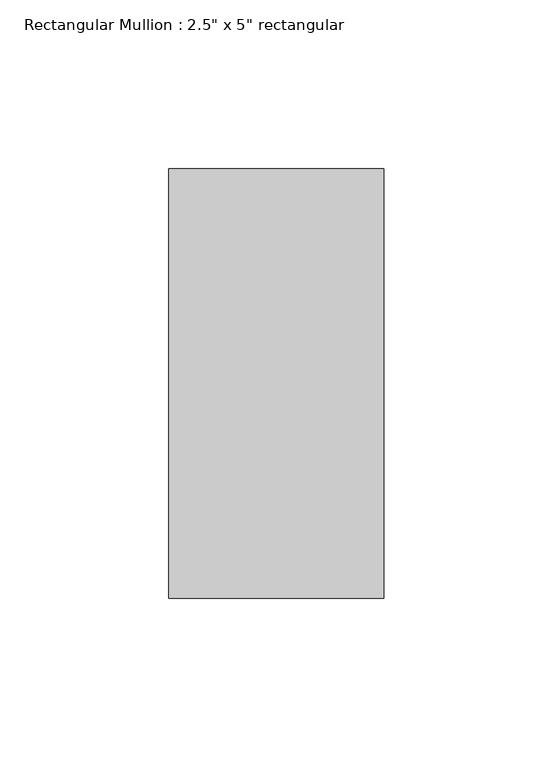
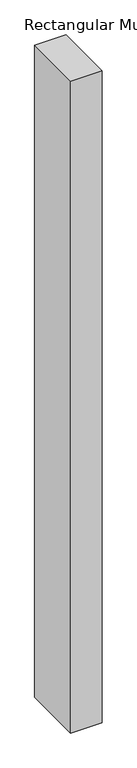
"""IFC4 building model written with IfcOpenShell, lengths in millimetres: member geometry."""

from ifc_helpers import new_model, si_unit, frame, origin, place, context, project, spatial, polyline, outline, extrude, source, transform, mapped, element, save


def member_a7a962ec(model_context):
    return source(origin(), model_context, "Body", "SweptSolid", [
        extrude(outline(polyline([(31.75, 63.5), (31.75, -63.5), (-31.75, -63.5), (-31.75, 63.5), (31.75, 63.5)])), frame((0.0, 0.0, -1401.633189), z_axis=(0.0, 0.0, 1.0), x_axis=(1.0, 0.0, 0.0)), (0.0, 0.0, 1.0), 1401.633189),
    ])


if __name__ == "__main__":
    model = new_model("IFC4")
    model_context = context("Model", 3, world=origin())
    ifc_project = project(units=[si_unit("LENGTHUNIT", "METRE", prefix="MILLI")], contexts=[model_context])
    site = spatial("IfcSite", under=ifc_project)
    building = spatial("IfcBuilding", under=site)
    placement = place(None, origin())
    member_shape = member_a7a962ec(model_context)
    element("IfcMember", 1, ObjectType="Rectangular Mullion : 2.5\" x 5\" rectangular", at=placement, inside=building, context=model_context, shape_type="MappedRepresentation", body=[
        mapped(member_shape, transform((0.0, 0.0, 0.0), x_axis=(1.0, 0.0, 0.0), y_axis=(0.0, 1.0, 0.0), z_axis=(0.0, 0.0, 1.0))),
    ])
    save(model, "model.ifc")

# Revit data of these elements
# Type "Rectangular Mullion : 2.5\" x 5\" rectangular"
#   built-in parameter 1007304 = 0.416667 (stored number, unit not read)
#   built-in parameter 1007301 = 0.104167 (stored number, unit not read)
#   built-in parameter 1007300 = 0.104167 (stored number, unit not read)
# Element 1 (IfcMember, "Rectangular Mullion : 2.5\" x 5\" rectangular")
#   Materials on its faces: "Aluminum"
# Materials
#   "Aluminum": class "Metal", colour RGB 247 247 247, transparency 0, Description = "Aluminum 6061", Cost = 0
